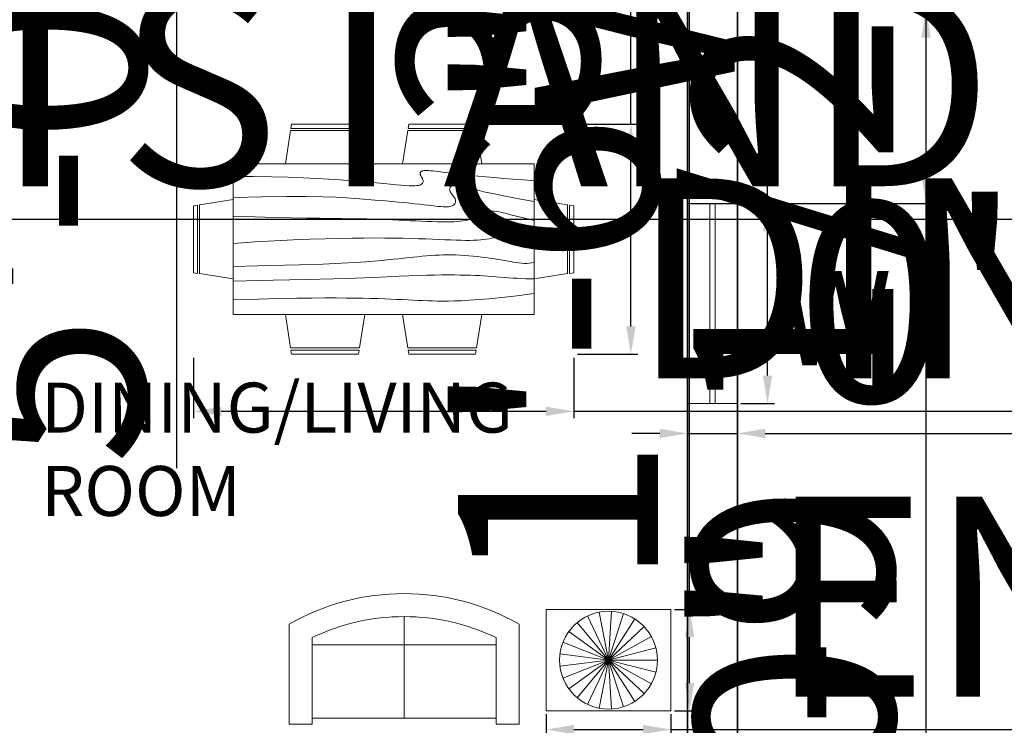
# Model space of a CAD drawing. Units: inches. Extents: x 2901 to 21549, y 2042 to 3828.
# Tile 5 of 10: x 3505 to 3682, y 3099 to 3226. Entities that reach past the tile are written whole.
import ezdxf

# ---------------------------------------------------------------- set-up
doc = ezdxf.new("R2010")
doc.units = ezdxf.units.IN
doc.layers.get('Defpoints').update_dxf_attribs({"color": 1})
for name, color, linetype, lineweight in [('A-ANNO-DIMS', 2, 'Continuous', 18), ('A-ANNO-TEXT', 7, 'Continuous', 18), ('A-AREA-IDEN', 7, 'Continuous', 18), ('A-FURN', 8, 'Continuous', 18), ('A-GLAZ', 4, 'Continuous', 18), ('A-WALL', 7, 'Continuous', 35)]:
    doc.layers.add(name, color=color, linetype=linetype, lineweight=lineweight)
doc.styles.get("Standard").update_dxf_attribs({"font": 'arial.ttf'})
doc.dimstyles.new('ISO-25', dxfattribs={"dimtxt": 36, "dimasz": 5, "dimexe": 1.25, "dimexo": 0.625, "dimtad": 1, "dimdec": 0, "dimlunit": 3, "dimtxsty": 'Standard', "dimcen": 2.5, "dimadec": 0, "dimazin": 0, "dimtfac": 1, "dimtdec": 0, "dimtmove": 0, "dimatfit": 3, "dimfxl": 1, "dimarcsym": 0})

# ---------------------------------------------------------------- blocks, each defined once
blk = doc.blocks.new('Dining Set - 36 x 72 in.')
for p, q in [((-22.2343, 26.00059), (-23.4847, 17.99762)), ((-22.2304, 26), (-5.7608, 26)), ((-22, 27.5), (-22.1562, 26.50042)), ((-5.8416, 26.5), (-22.1534, 26.5)), ((-22, 27.5), (-6, 27.5)), ((-5.8437, 26.49966), (-6, 27.5)), ((-4.5152, 17.99762), (-5.7655, 25.99926)), ((5.7657, 26.00059), (4.5153, 17.99762)), ((5.7696, 26), (22.2392, 26)), ((6, 27.5), (5.8438, 26.50042)), ((22.1584, 26.5), (5.8466, 26.5)), ((6, 27.5), (22, 27.5)), ((22.1563, 26.49966), (22, 27.5)), ((23.4848, 17.99762), (22.2345, 25.99926)), ((36, 18), (-36, 18)), ((-36, 18), (-36, -18)), ((36, -18), (36, 18)), ((-44.0006, 8.23428), (-35.9976, 9.48474)), ((44.0006, 8.23428), (35.9976, 9.48474)), ((-45.5, 8), (-44.5004, 8.15617)), ((-45.5, 8), (-45.5, -8)), ((-44.5, -8.15843), (-44.5, 8.15338)), ((-44, 8.23041), (-44, -8.23915)), ((44, 8.23041), (44, -8.23915)), ((44.5, -8.15843), (44.5, 8.15338)), ((45.5, 8), (44.5005, 8.15617)), ((45.5, 8), (45.5, -8)), ((-44.4997, -8.15631), (-45.5, -8)), ((-35.9976, -9.48476), (-43.9993, -8.2345)), ((35.9976, -9.48476), (43.9993, -8.2345)), ((44.4997, -8.15631), (45.5, -8)), ((-36, -18), (36, -18)), ((-22.2343, -26.0006), (-23.4847, -17.99762)), ((-4.5152, -17.99762), (-5.7655, -25.99928)), ((5.7657, -26.0006), (4.5153, -17.99762)), ((23.4848, -17.99762), (22.2345, -25.99928)), ((-22.2304, -26), (-5.7608, -26)), ((-22, -27.5), (-22.1562, -26.50044)), ((-5.8416, -26.5), (-22.1534, -26.5)), ((-22, -27.5), (-6, -27.5)), ((-5.8437, -26.49967), (-6, -27.5)), ((5.7696, -26), (22.2392, -26)), ((6, -27.5), (5.8438, -26.50044)), ((22.1584, -26.5), (5.8466, -26.5)), ((6, -27.5), (22, -27.5)), ((22.1563, -26.49967), (22, -27.5))]:
    blk.add_line(p, q)
for points in [[(-36, 15), (-31.1772, 14.97754), (-26.8079, 14.91406), (-22.8538, 14.81543), (-19.276, 14.6875), (-16.0362, 14.53613), (-13.0957, 14.36718), (-10.4159, 14.18652), (-7.9583, 14), (-5.6904, 13.81315), (-3.6035, 13.63021), (-1.6954, 13.45508), (0.0365, 13.29166), (1.5945, 13.14388), (2.9811, 13.01562), (4.1988, 12.9108), (5.25, 12.83333), (6.1393, 12.78613), (6.8802, 12.76823), (7.4883, 12.77767), (7.9792, 12.8125), (8.3685, 12.87077), (8.6719, 12.95052), (8.9049, 13.0498), (9.0833, 13.16666), (9.2205, 13.29899), (9.3216, 13.44401), (9.3895, 13.59879), (9.4271, 13.76041), (9.4373, 13.92594), (9.4232, 14.09245), (9.3875, 14.257), (9.3333, 14.41666), (9.2638, 14.56917), (9.1836, 14.71484), (9.0975, 14.85465), (9.0104, 14.98958), (8.9272, 15.1206), (8.8529, 15.2487), (8.7922, 15.37483), (8.75, 15.5), (8.7305, 15.62467), (8.7344, 15.74739), (8.7617, 15.86621), (8.8125, 15.97916), (8.8867, 16.08431), (8.9844, 16.17968), (9.1055, 16.26334), (9.25, 16.33333), (9.4189, 16.38802), (9.6172, 16.42708), (9.8506, 16.45052), (10.125, 16.45833), (10.4463, 16.45052), (10.8203, 16.42708), (11.2529, 16.38802), (11.75, 16.33333), (12.3184, 16.26318), (12.9694, 16.17838), (13.7151, 16.07991), (14.5677, 15.96875), (15.5395, 15.84586), (16.6426, 15.71224), (17.8893, 15.56884), (19.2917, 15.41666), (20.859, 15.25667), (22.5879, 15.08984), (24.4721, 14.91715), (26.5052, 14.73958), (28.6809, 14.5581), (30.9929, 14.3737), (33.4347, 14.18733), (36, 14)], [(-36, 10), (-28.9766, 10.14274), (-23.1725, 10.20442), (-18.4241, 10.19775), (-14.5677, 10.13541), (-11.4399, 10.03011), (-8.877, 9.89453), (-6.7154, 9.74137), (-4.7917, 9.58333), (-2.9698, 9.43082), (-1.2246, 9.28515), (0.4415, 9.14534), (2.026, 9.01041), (3.5266, 8.87939), (4.9408, 8.7513), (6.266, 8.62516), (7.5, 8.5), (8.6411, 8.37549), (9.6914, 8.2539), (10.6538, 8.13818), (11.5312, 8.03125), (12.3267, 7.93603), (13.043, 7.85547), (13.6831, 7.79248), (14.25, 7.75), (14.7471, 7.7303), (15.1797, 7.73307), (15.5537, 7.75732), (15.875, 7.80208), (16.1494, 7.86637), (16.3828, 7.94922), (16.5811, 8.04964), (16.75, 8.16666), (16.8944, 8.29915), (17.0143, 8.44531), (17.1089, 8.60319), (17.1771, 8.77083), (17.218, 8.94629), (17.2305, 9.1276), (17.2137, 9.31282), (17.1667, 9.5), (17.0895, 9.6875), (16.987, 9.875), (16.8649, 10.0625), (16.7292, 10.25), (16.5856, 10.4375), (16.4401, 10.625), (16.2985, 10.8125), (16.1667, 11), (16.05, 11.18733), (15.9518, 11.3737), (15.8752, 11.5581), (15.8229, 11.73958), (15.798, 11.91715), (15.8034, 12.08984), (15.842, 12.25667), (15.9167, 12.41666), (16.0295, 12.56836), (16.1784, 12.70833), (16.3605, 12.83268), (16.5729, 12.9375), (16.8127, 13.01888), (17.0768, 13.07291), (17.3625, 13.0957), (17.6667, 13.08333), (17.9894, 13.03312), (18.3418, 12.94726), (18.7382, 12.82918), (19.1927, 12.68229), (19.7195, 12.51001), (20.3327, 12.31575), (21.0465, 12.10294), (21.875, 11.875), (22.8357, 11.63354), (23.959, 11.37304), (25.2786, 11.08618), (26.8282, 10.76562), (28.6414, 10.40405), (30.752, 9.99414), (33.1936, 9.52856), (36, 9)], [(-36, 5.5), (-30.7157, 5.3348), (-26.069, 5.20963), (-21.9946, 5.11767), (-18.4271, 5.05208), (-15.3009, 5.00602), (-12.5508, 4.97265), (-10.1112, 4.94515), (-7.9167, 4.91666), (-5.909, 4.88167), (-4.0586, 4.83984), (-2.3429, 4.79215), (-0.7396, 4.73958), (0.7739, 4.6831), (2.22, 4.6237), (3.6213, 4.56233), (5, 4.5), (6.373, 4.43782), (7.7344, 4.3776), (9.0723, 4.32129), (10.375, 4.27083), (11.6309, 4.22819), (12.8281, 4.19531), (13.9551, 4.17415), (15, 4.16666), (15.954, 4.17448), (16.819, 4.19791), (17.6001, 4.23698), (18.3021, 4.29166), (18.9299, 4.36198), (19.4883, 4.44791), (19.9823, 4.54948), (20.4167, 4.66666), (20.7969, 4.79899), (21.1302, 4.94401), (21.4245, 5.09879), (21.6875, 5.26041), (21.9271, 5.42594), (22.1511, 5.59245), (22.3672, 5.757), (22.5834, 5.91666), (22.8065, 6.06868), (23.0404, 6.21093), (23.2879, 6.34147), (23.5521, 6.45833), (23.8358, 6.55957), (24.142, 6.64323), (24.4735, 6.70735), (24.8334, 6.75), (25.2235, 6.76969), (25.642, 6.76692), (26.0858, 6.74267), (26.5521, 6.69791), (27.0379, 6.63362), (27.5404, 6.55078), (28.0565, 6.45036), (28.5834, 6.33333), (29.1242, 6.19987), (29.7071, 6.04687), (30.3661, 5.87044), (31.1354, 5.66666), (32.0493, 5.43164), (33.142, 5.16146), (34.4475, 4.85221), (36, 4.5)], [(-36, -1), (-30.7915, -0.6591), (-26.0195, -0.38216), (-21.6519, -0.16284), (-17.6563, 0.00521), (-14.0005, 0.12833), (-10.6523, 0.21289), (-7.5796, 0.26522), (-4.75, 0.29166), (-2.134, 0.29793), (0.2878, 0.28711), (2.5317, 0.26163), (4.6146, 0.22396), (6.5529, 0.17651), (8.3633, 0.12174), (10.0623, 0.06209), (11.6667, 0), (13.1899, -0.06201), (14.6341, -0.1211), (15.9982, -0.17432), (17.2813, -0.21875), (18.4823, -0.25147), (19.6003, -0.26953), (20.6343, -0.27002), (21.5834, -0.25), (22.4481, -0.20768), (23.2357, -0.14584), (23.9549, -0.06836), (24.6146, 0.02083), (25.2235, 0.11784), (25.7904, 0.21875), (26.3241, 0.31966), (26.8334, 0.41666), (27.3265, 0.50618), (27.8099, 0.58593), (28.2894, 0.65397), (28.7709, 0.70833), (29.2601, 0.74707), (29.763, 0.76823), (30.2855, 0.76985), (30.8334, 0.75), (31.4088, 0.70784), (31.9994, 0.64713), (32.589, 0.57275), (33.1615, 0.48958), (33.7008, 0.4025), (34.1908, 0.3164), (34.6153, 0.23616), (34.9584, 0.16666), (35.2099, 0.11165), (35.3848, 0.07031), (35.504, 0.04069), (35.5886, 0.02083), (35.6594, 0.00879), (35.7377, 0.0026), (35.8442, 0.00032), (36, 0)], [(-36, -6.5), (-27.1843, -6.31267), (-20.084, -6.1263), (-14.469, -5.9419), (-10.1094, -5.76042), (-6.7752, -5.58285), (-4.2363, -5.41016), (-2.2629, -5.24333), (-0.625, -5.08334), (0.8708, -4.93099), (2.2715, -4.78646), (3.5872, -4.64974), (4.8281, -4.52084), (6.0046, -4.39974), (7.127, -4.28646), (8.2053, -4.18099), (9.25, -4.08334), (10.2705, -3.99382), (11.2734, -3.91407), (12.2647, -3.84603), (13.25, -3.79167), (14.2354, -3.75293), (15.2266, -3.73177), (16.2295, -3.73015), (17.25, -3.75), (18.2912, -3.79248), (19.3451, -3.85547), (20.4009, -3.93604), (21.4479, -4.03125), (22.4754, -4.13819), (23.4727, -4.25391), (24.4289, -4.37549), (25.3334, -4.5), (26.1785, -4.62492), (26.9694, -4.74935), (27.7145, -4.87281), (28.4219, -4.99479), (29.1, -5.11483), (29.7572, -5.23242), (30.4016, -5.34709), (31.0417, -5.45834), (31.6837, -5.56437), (32.3262, -5.65821), (32.9658, -5.73153), (33.599, -5.77604), (34.2224, -5.78345), (34.8327, -5.74545), (35.4264, -5.65373), (36, -5.5)], [(-36, -10), (-26.4022, -9.81299), (-18.4675, -9.62891), (-11.9839, -9.45069), (-6.7396, -9.28125), (-2.5226, -9.12354), (0.8789, -8.98047), (3.6769, -8.85498), (6.0833, -8.75), (8.2767, -8.66765), (10.3021, -8.60677), (12.1712, -8.56543), (13.8958, -8.54167), (15.4876, -8.53353), (16.9583, -8.53907), (18.3197, -8.55632), (19.5834, -8.58334), (20.7616, -8.61841), (21.8685, -8.66081), (22.9188, -8.71004), (23.9271, -8.76563), (24.9081, -8.82707), (25.8763, -8.89388), (26.8465, -8.96558), (27.8334, -9.04167), (28.8474, -9.12118), (29.8828, -9.20117), (30.93, -9.27824), (31.9792, -9.34896), (33.0205, -9.40991), (34.0443, -9.45768), (35.0407, -9.48885), (36, -9.5)], [(-36, -14.5), (-30.0881, -14.33513), (-25.0332, -14.21224), (-20.7312, -14.12647), (-17.0781, -14.07292), (-13.97, -14.04671), (-11.3027, -14.04297), (-8.9724, -14.05681), (-6.875, -14.08334), (-4.9224, -14.11833), (-3.0905, -14.16016), (-1.3709, -14.20785), (0.2448, -14.26042), (1.7647, -14.3169), (3.1973, -14.3763), (4.5507, -14.43767), (5.8333, -14.5), (7.0554, -14.5621), (8.235, -14.62175), (9.3922, -14.67652), (10.5469, -14.72396), (11.7192, -14.76164), (12.929, -14.78711), (14.1965, -14.79794), (15.5417, -14.79167), (16.9933, -14.76424), (18.6152, -14.70508), (20.4804, -14.60197), (22.6615, -14.44271), (25.2312, -14.21509), (28.2624, -13.9069), (31.8277, -13.50594), (36, -13)]]:
    blk.add_lwpolyline(points)
blk = doc.blocks.new('Sofa - Roundback Loveseat 5 ft.')
for p, q in [((0, -32.44198), (0, -5.99998)), ((-24, -33.99998), (-24, -11.46958)), ((24.00004, -33.99998), (24.00004, -11.46958)), ((-23.9998, -13.38178), (23.99986, -13.38178)), ((-24, -32.44198), (24.00004, -32.44198))]:
    blk.add_line(p, q)
for points in [[(-24, -33.99998), (-30, -33.99998), (-30, -7.99998)], [(30.00004, -7.99998), (30.00004, -33.99998), (24.00004, -33.99998)]]:
    blk.add_lwpolyline(points)
for centre, radius, start, end in [((0, -60.24998), 60.24998, 60.13715, 119.8628), ((0, -61.38438), 55.38444, 64.32083, 115.6792)]:
    blk.add_arc(centre, radius, start, end)
blk = doc.blocks.new('WIN-36IN-9IN-WALL')
for p, q in [((0, 36), (9, 36)), ((0, 0), (0, 36)), ((4, 0), (4, 36)), ((5, 36), (5, 0)), ((9, 36), (9, 0)), ((9, 0), (0, 0))]:
    blk.add_line(p, q)
blk = doc.blocks.new('*U24')
blk.add_line((-4.41, 0), (4.41, 0))
blk = doc.blocks.new('*U25')
at = {"color": 0, "linetype": 'ByBlock', "lineweight": -2, "transparency": 16777216}
for p, rotation in [((3610.1, 3028.89), 100.7999999999996), ((3611.21, 3028.96), 86.39999999999972), ((3612.29, 3028.76), 71.99999999999977), ((3608.12, 3027.96), 129.5999999999996), ((3609.05, 3028.55), 115.1999999999997), ((3613.29, 3028.29), 57.59999999999982), ((3607.36, 3027.15), 143.9999999999996), ((3614.14, 3027.58), 43.19999999999986), ((3606.83, 3026.19), 158.3999999999996), ((3614.79, 3026.69), 28.7999999999999), ((3615.2, 3025.66), 14.39999999999998), ((3606.56, 3025.12), 172.7999999999996), ((3606.56, 3024.01), 187.1999999999994), ((3606.83, 3022.94), 201.5999999999995), ((3607.36, 3021.97), 215.9999999999995), ((3608.12, 3021.17), 230.3999999999995), ((3609.05, 3020.58), 244.7999999999995), ((3610.1, 3020.23), 259.1999999999994), ((3611.21, 3020.17), 273.5999999999994), ((3612.29, 3020.37), 287.9999999999993), ((3613.29, 3020.84), 302.3999999999992), ((3614.14, 3021.55), 316.7999999999993), ((3614.79, 3022.44), 331.1999999999992), ((3615.2, 3023.47), 345.5999999999992)]:
    blk.add_blockref('*U24', p, dxfattribs=dict(at, rotation=rotation))
blk.add_blockref('*U24', (3615.34, 3024.56), dxfattribs=at)
blk = doc.blocks.new('TABLE-END-DECOR')
blk.add_lwpolyline([(0, 18.24), (22.47, 18.24), (22.47, 0), (0, 0)], close=True)
blk.add_circle((11.23, 9.12), 8.81)
blk.add_blockref('*U25', (-3599.7, -3015.44))
blk = doc.blocks.new('*D36')
at = {"layer": 'A-ANNO-DIMS', "color": 0, "lineweight": -2, "transparency": 16777216}
for p, q in [((3639.47, 3192.64), (3639.47, 3654.44)), ((3634.69, 3192.64), (3640.72, 3192.64)), ((3639.47, 3161.64), (3639.47, 3187.64)), ((3634.69, 3156.64), (3640.72, 3156.64))]:
    blk.add_line(p, q, dxfattribs=at)
at = {"layer": 'A-ANNO-DIMS', "color": 0, "transparency": 16777216}
for points in [[(3638.64, 3187.64), (3640.3, 3187.64), (3639.47, 3192.64)], [(3638.64, 3161.64), (3640.3, 3161.64), (3639.47, 3156.64)]]:
    blk.add_solid(points, dxfattribs=at)
at = {"layer": 'Defpoints', "color": 0, "transparency": 16777216}
for p in [(3634.07, 3192.64), (3639.47, 3192.64), (3634.07, 3156.64)]:
    blk.add_point(p, dxfattribs=at)
at = {"layer": 'A-ANNO-DIMS', "color": 0, "transparency": 16777216, "insert": (3620.21, 3426.04), "char_height": 36, "attachment_point": 5, "rotation": 90}
blk.add_mtext('WINDOW 3\'-0" TYP.', dxfattribs=at)
blk = doc.blocks.new('*D37')
at = {"layer": 'A-ANNO-DIMS', "color": 0, "lineweight": -2, "transparency": 16777216}
for p, q in [((3625.07, 3156.01), (3625.07, 3149.99)), ((3634.07, 3156.01), (3634.07, 3149.99)), ((3620.07, 3151.24), (3615.07, 3151.24)), ((3625.07, 3151.24), (3634.07, 3151.24)), ((3639.07, 3151.24), (3864.76, 3151.24))]:
    blk.add_line(p, q, dxfattribs=at)
at = {"layer": 'A-ANNO-DIMS', "color": 0, "transparency": 16777216}
for points in [[(3620.07, 3152.07), (3620.07, 3150.41), (3625.07, 3151.24)], [(3639.07, 3152.07), (3639.07, 3150.41), (3634.07, 3151.24)]]:
    blk.add_solid(points, dxfattribs=at)
at = {"layer": 'Defpoints', "color": 0, "transparency": 16777216}
for p in [(3625.07, 3156.64), (3634.07, 3156.64), (3634.07, 3151.24)]:
    blk.add_point(p, dxfattribs=at)
at = {"layer": 'A-ANNO-DIMS', "color": 0, "transparency": 16777216, "insert": (3754.41, 3170.24), "char_height": 36, "attachment_point": 5}
blk.add_mtext('0\'-9" TYP.', dxfattribs=at)
blk = doc.blocks.new('*D38')
at = {"layer": 'A-ANNO-DIMS', "color": 0, "lineweight": -2, "transparency": 16777216}
for p, q in [((3343.07, 3191.34), (3343.07, 3188.58)), ((3357.29, 3191.34), (3357.29, 3188.58)), ((3348.07, 3189.83), (3352.29, 3189.83)), ((3357.29, 3189.83), (3922.11, 3189.83))]:
    blk.add_line(p, q, dxfattribs=at)
at = {"layer": 'A-ANNO-DIMS', "color": 0, "transparency": 16777216}
for points in [[(3348.07, 3190.67), (3348.07, 3189), (3343.07, 3189.83)], [(3352.29, 3190.67), (3352.29, 3189), (3357.29, 3189.83)]]:
    blk.add_solid(points, dxfattribs=at)
at = {"layer": 'Defpoints', "color": 0, "transparency": 16777216}
for p in [(3343.07, 3191.97), (3357.29, 3191.97), (3357.29, 3189.83)]:
    blk.add_point(p, dxfattribs=at)
at = {"layer": 'A-ANNO-DIMS', "color": 0, "transparency": 16777216, "insert": (3642.2, 3209.07), "char_height": 36, "attachment_point": 5}
blk.add_mtext('NIGHTSTAND 1\'-2" TYP.', dxfattribs=at)
blk = doc.blocks.new('*D43')
at = {"layer": 'A-ANNO-DIMS', "color": 0, "lineweight": -2, "transparency": 16777216}
for p, q in [((3550.8, 3269.4), (3856.95, 3274.04)), ((3536.1, 3267.11), (3536.05, 3270.42)), ((3550.83, 3267.33), (3550.78, 3270.65)), ((3541.07, 3269.25), (3545.8, 3269.32))]:
    blk.add_line(p, q, dxfattribs=at)
at = {"layer": 'A-ANNO-DIMS', "color": 0, "transparency": 16777216}
for points in [[(3541.06, 3270.08), (3541.09, 3268.42), (3536.07, 3269.17)], [(3545.78, 3270.16), (3545.81, 3268.49), (3550.8, 3269.4)]]:
    blk.add_solid(points, dxfattribs=at)
at = {"layer": 'Defpoints', "color": 0, "transparency": 16777216}
for p in [(3550.8, 3269.4), (3536.11, 3266.48), (3550.84, 3266.71)]:
    blk.add_point(p, dxfattribs=at)
at = {"layer": 'A-ANNO-DIMS', "color": 0, "transparency": 16777216, "insert": (3706.08, 3290.99), "char_height": 36, "attachment_point": 5, "rotation": 0.8679}
blk.add_mtext('1\'-2 1/2" TYP.', dxfattribs=at)
blk = doc.blocks.new('*D47')
at = {"layer": 'A-ANNO-DIMS', "color": 0, "lineweight": -2, "transparency": 16777216}
for p, q in [((3544.44, 3430.67), (3531.82, 3430.67)), ((3533.07, 3425.67), (3533.07, 3375.67)), ((3544.44, 3370.67), (3531.82, 3370.67)), ((3533.07, 3370.67), (3533.07, 3144.99))]:
    blk.add_line(p, q, dxfattribs=at)
at = {"layer": 'A-ANNO-DIMS', "color": 0, "transparency": 16777216}
for points in [[(3532.24, 3425.67), (3533.9, 3425.67), (3533.07, 3430.67)], [(3532.24, 3375.67), (3533.9, 3375.67), (3533.07, 3370.67)]]:
    blk.add_solid(points, dxfattribs=at)
at = {"layer": 'Defpoints', "color": 0, "transparency": 16777216}
for p in [(3545.07, 3430.67), (3533.07, 3370.67), (3545.07, 3370.67)]:
    blk.add_point(p, dxfattribs=at)
at = {"layer": 'A-ANNO-DIMS', "color": 0, "transparency": 16777216, "insert": (3514.06, 3255.33), "char_height": 36, "attachment_point": 5, "rotation": 90}
blk.add_mtext('5\'-0" TYP.', dxfattribs=at)
blk = doc.blocks.new('*D48')
at = {"layer": 'A-ANNO-DIMS', "color": 0, "lineweight": -2, "transparency": 16777216}
for p, q in [((3552.33, 3036.58), (3552.33, 3043.43)), ((3557.33, 3042.18), (3588.77, 3042.18)), ((3593.77, 3036.58), (3593.77, 3043.43)), ((3593.77, 3042.18), (4181.25, 3042.18))]:
    blk.add_line(p, q, dxfattribs=at)
at = {"layer": 'A-ANNO-DIMS', "color": 0, "transparency": 16777216}
for points in [[(3557.33, 3043.01), (3557.33, 3041.34), (3552.33, 3042.18)], [(3588.77, 3043.01), (3588.77, 3041.34), (3593.77, 3042.18)]]:
    blk.add_solid(points, dxfattribs=at)
at = {"layer": 'Defpoints', "color": 0, "transparency": 16777216}
for p in [(3593.77, 3042.18), (3552.33, 3035.96), (3593.77, 3035.96)]:
    blk.add_point(p, dxfattribs=at)
at = {"layer": 'A-ANNO-DIMS', "color": 0, "transparency": 16777216, "insert": (3890.01, 3061.44), "char_height": 36, "attachment_point": 5}
blk.add_mtext('LOVESEAT 3\'-5 1/2" TYP.', dxfattribs=at)
blk = doc.blocks.new('*D50')
at = {"layer": 'A-ANNO-DIMS', "color": 0, "lineweight": -2, "transparency": 16777216}
for p, q in [((3599.61, 3100.68), (3599.61, 3096.69)), ((3622.08, 3100.68), (3622.08, 3096.69)), ((3604.61, 3097.94), (3617.08, 3097.94)), ((3622.08, 3097.94), (4251.18, 3097.94))]:
    blk.add_line(p, q, dxfattribs=at)
at = {"layer": 'A-ANNO-DIMS', "color": 0, "transparency": 16777216}
for points in [[(3604.61, 3098.77), (3604.61, 3097.1), (3599.61, 3097.94)], [(3617.08, 3098.77), (3617.08, 3097.1), (3622.08, 3097.94)]]:
    blk.add_solid(points, dxfattribs=at)
at = {"layer": 'Defpoints', "color": 0, "transparency": 16777216}
for p in [(3599.61, 3101.31), (3622.08, 3101.31), (3622.08, 3097.94)]:
    blk.add_point(p, dxfattribs=at)
at = {"layer": 'A-ANNO-DIMS', "color": 0, "transparency": 16777216, "insert": (3939.13, 3117.18), "char_height": 36, "attachment_point": 5}
blk.add_mtext('END TABLE 1\'-10 1/2" TYP.', dxfattribs=at)
blk = doc.blocks.new('*D51')
at = {"layer": 'A-ANNO-DIMS', "color": 0, "lineweight": -2, "transparency": 16777216}
for p, q in [((3625.45, 3119.55), (3625.45, 3341.85)), ((3622.7, 3119.55), (3626.7, 3119.55)), ((3625.45, 3106.31), (3625.45, 3114.55)), ((3622.7, 3101.31), (3626.7, 3101.31))]:
    blk.add_line(p, q, dxfattribs=at)
at = {"layer": 'A-ANNO-DIMS', "color": 0, "transparency": 16777216}
for points in [[(3624.61, 3114.55), (3626.28, 3114.55), (3625.45, 3119.55)], [(3624.61, 3106.31), (3626.28, 3106.31), (3625.45, 3101.31)]]:
    blk.add_solid(points, dxfattribs=at)
at = {"layer": 'Defpoints', "color": 0, "transparency": 16777216}
for p in [(3622.08, 3119.55), (3625.45, 3119.55), (3622.08, 3101.31)]:
    blk.add_point(p, dxfattribs=at)
at = {"layer": 'A-ANNO-DIMS', "color": 0, "transparency": 16777216, "insert": (3606.44, 3233.2), "char_height": 36, "attachment_point": 5, "rotation": 90}
blk.add_mtext('1\'-6" TYP.', dxfattribs=at)
blk = doc.blocks.new('*D52')
at = {"layer": 'A-ANNO-DIMS', "color": 0, "lineweight": -2, "transparency": 16777216}
for p, q in [((3469.26, 3197.35), (3456.81, 3197.35)), ((3458.06, 3192.35), (3458.06, 3123.52)), ((3469.26, 3118.52), (3456.81, 3118.52)), ((3458.06, 3118.52), (3458.06, 2589.92))]:
    blk.add_line(p, q, dxfattribs=at)
at = {"layer": 'A-ANNO-DIMS', "color": 0, "transparency": 16777216}
for points in [[(3457.23, 3192.35), (3458.9, 3192.35), (3458.06, 3197.35)], [(3457.23, 3123.52), (3458.9, 3123.52), (3458.06, 3118.52)]]:
    blk.add_solid(points, dxfattribs=at)
at = {"layer": 'Defpoints', "color": 0, "transparency": 16777216}
for p in [(3469.89, 3197.35), (3458.06, 3118.52), (3469.89, 3118.52)]:
    blk.add_point(p, dxfattribs=at)
at = {"layer": 'A-ANNO-DIMS', "color": 0, "transparency": 16777216, "insert": (3439.06, 2851.72), "char_height": 36, "attachment_point": 5, "rotation": 90}
blk.add_mtext('MEDIA UNIT 6\'-7" TYP.', dxfattribs=at)
blk = doc.blocks.new('*D54')
at = {"layer": 'A-ANNO-DIMS', "color": 0, "lineweight": -2, "transparency": 16777216}
for p, q in [((3536.12, 3164.87), (3536.12, 3153.97)), ((3604.61, 3164.87), (3604.61, 3153.97)), ((3541.12, 3155.22), (3599.61, 3155.22)), ((3604.61, 3155.22), (4090.43, 3155.22))]:
    blk.add_line(p, q, dxfattribs=at)
at = {"layer": 'A-ANNO-DIMS', "color": 0, "transparency": 16777216}
for points in [[(3541.12, 3156.05), (3541.12, 3154.38), (3536.12, 3155.22)], [(3599.61, 3156.05), (3599.61, 3154.38), (3604.61, 3155.22)]]:
    blk.add_solid(points, dxfattribs=at)
at = {"layer": 'Defpoints', "color": 0, "transparency": 16777216}
for p in [(3536.12, 3165.49), (3604.61, 3165.49), (3604.61, 3155.22)]:
    blk.add_point(p, dxfattribs=at)
at = {"layer": 'A-ANNO-DIMS', "color": 0, "transparency": 16777216, "insert": (3850.02, 3174.46), "char_height": 36, "attachment_point": 5}
blk.add_mtext('DINING SET 5\'-8 1/2"', dxfattribs=at)
blk = doc.blocks.new('*D55')
at = {"layer": 'A-ANNO-DIMS', "color": 0, "lineweight": -2, "transparency": 16777216}
for p, q in [((3614.88, 3206.89), (3614.88, 3392.69)), ((3605.24, 3206.89), (3616.13, 3206.89)), ((3614.88, 3170.49), (3614.88, 3201.89)), ((3605.24, 3165.49), (3616.13, 3165.49))]:
    blk.add_line(p, q, dxfattribs=at)
at = {"layer": 'A-ANNO-DIMS', "color": 0, "transparency": 16777216}
for points in [[(3614.05, 3201.89), (3615.72, 3201.89), (3614.88, 3206.89)], [(3614.05, 3170.49), (3615.72, 3170.49), (3614.88, 3165.49)]]:
    blk.add_solid(points, dxfattribs=at)
at = {"layer": 'Defpoints', "color": 0, "transparency": 16777216}
for p in [(3604.61, 3206.89), (3614.88, 3206.89), (3604.61, 3165.49)]:
    blk.add_point(p, dxfattribs=at)
at = {"layer": 'A-ANNO-DIMS', "color": 0, "transparency": 16777216, "insert": (3595.63, 3302.29), "char_height": 36, "attachment_point": 5, "rotation": 90}
blk.add_mtext('3\'-5 1/2"', dxfattribs=at)
blk = doc.blocks.new('*D57')
at = {"layer": 'A-ANNO-DIMS', "color": 0, "lineweight": -2, "transparency": 16777216}
for p, q in [((3601.59, 3038.97), (3601.59, 3029.64)), ((3626.91, 3038.97), (3626.91, 3029.64)), ((3606.59, 3030.89), (3621.91, 3030.89)), ((3626.91, 3030.89), (3813.36, 3030.89))]:
    blk.add_line(p, q, dxfattribs=at)
at = {"layer": 'A-ANNO-DIMS', "color": 0, "transparency": 16777216}
for points in [[(3606.59, 3031.73), (3606.59, 3030.06), (3601.59, 3030.89)], [(3621.91, 3031.73), (3621.91, 3030.06), (3626.91, 3030.89)]]:
    blk.add_solid(points, dxfattribs=at)
at = {"layer": 'Defpoints', "color": 0, "transparency": 16777216}
for p in [(3601.59, 3039.6), (3626.91, 3039.6), (3626.91, 3030.89)]:
    blk.add_point(p, dxfattribs=at)
at = {"layer": 'A-ANNO-DIMS', "color": 0, "transparency": 16777216, "insert": (3722.63, 3050.13), "char_height": 36, "attachment_point": 5}
blk.add_mtext('2\'-1 1/2"', dxfattribs=at)
blk = doc.blocks.new('*D65')
at = {"layer": 'A-ANNO-DIMS', "color": 0, "lineweight": -2, "transparency": 16777216}
for p, q in [((3668.02, 3003.48), (3668.02, 3130.01)), ((3625.69, 3003.48), (3669.27, 3003.48)), ((3668.02, 2888.48), (3668.02, 2998.48)), ((3625.69, 2883.48), (3669.27, 2883.48))]:
    blk.add_line(p, q, dxfattribs=at)
at = {"layer": 'A-ANNO-DIMS', "color": 0, "transparency": 16777216}
for points in [[(3667.19, 2998.48), (3668.85, 2998.48), (3668.02, 3003.48)], [(3667.19, 2888.48), (3668.85, 2888.48), (3668.02, 2883.48)]]:
    blk.add_solid(points, dxfattribs=at)
at = {"layer": 'Defpoints', "color": 0, "transparency": 16777216}
for p in [(3625.07, 3003.48), (3668.02, 3003.48), (3625.07, 2883.48)]:
    blk.add_point(p, dxfattribs=at)
at = {"layer": 'A-ANNO-DIMS', "color": 0, "transparency": 16777216, "insert": (3649.01, 3069.24), "char_height": 36, "attachment_point": 5, "rotation": 90}
blk.add_mtext('10\'-0"', dxfattribs=at)
blk = doc.blocks.new('*D67')
at = {"layer": 'A-ANNO-DIMS', "color": 0, "lineweight": -2, "transparency": 16777216}
for p, q in [((3484.07, 3013.1), (3484.07, 3509.68)), ((3489.07, 3508.43), (3620.07, 3508.43)), ((3625.07, 3228.1), (3625.07, 3509.68))]:
    blk.add_line(p, q, dxfattribs=at)
at = {"layer": 'A-ANNO-DIMS', "color": 0, "transparency": 16777216}
for points in [[(3489.07, 3509.26), (3489.07, 3507.59), (3484.07, 3508.43)], [(3620.07, 3509.26), (3620.07, 3507.59), (3625.07, 3508.43)]]:
    blk.add_solid(points, dxfattribs=at)
at = {"layer": 'Defpoints', "color": 0, "transparency": 16777216}
for p in [(3625.07, 3508.43), (3625.07, 3227.48), (3484.07, 3012.48)]:
    blk.add_point(p, dxfattribs=at)
at = {"layer": 'A-ANNO-DIMS', "color": 0, "transparency": 16777216, "insert": (3554.57, 3527.43), "char_height": 36, "attachment_point": 5}
blk.add_mtext('11\'-9"', dxfattribs=at)
blk = doc.blocks.new('*D68')
at = {"layer": 'A-ANNO-DIMS', "color": 0, "lineweight": -2, "transparency": 16777216}
for p, q in [((3531.44, 3227.48), (3298.87, 3227.48)), ((3300.12, 3017.48), (3300.12, 3222.48)), ((3483.44, 3012.48), (3298.87, 3012.48))]:
    blk.add_line(p, q, dxfattribs=at)
at = {"layer": 'A-ANNO-DIMS', "color": 0, "transparency": 16777216}
for points in [[(3299.29, 3222.48), (3300.95, 3222.48), (3300.12, 3227.48)], [(3299.29, 3017.48), (3300.95, 3017.48), (3300.12, 3012.48)]]:
    blk.add_solid(points, dxfattribs=at)
at = {"layer": 'Defpoints', "color": 0, "transparency": 16777216}
for p in [(3300.12, 3227.48), (3532.07, 3227.48), (3484.07, 3012.48)]:
    blk.add_point(p, dxfattribs=at)
at = {"layer": 'A-ANNO-DIMS', "color": 0, "transparency": 16777216, "insert": (3281.42, 3119.98), "char_height": 36, "attachment_point": 5, "rotation": 90}
blk.add_mtext('17\'-11"', dxfattribs=at)
blk = doc.blocks.new('*D73')
at = {"layer": 'A-ANNO-DIMS', "color": 0, "lineweight": -2, "transparency": 16777216}
for p, q in [((3668.02, 3058.19), (3668.02, 3244)), ((3625.69, 3058.19), (3669.27, 3058.19)), ((3668.02, 3017.48), (3668.02, 3053.19)), ((3625.69, 3012.48), (3669.27, 3012.48))]:
    blk.add_line(p, q, dxfattribs=at)
at = {"layer": 'A-ANNO-DIMS', "color": 0, "transparency": 16777216}
for points in [[(3667.19, 3053.19), (3668.85, 3053.19), (3668.02, 3058.19)], [(3667.19, 3017.48), (3668.85, 3017.48), (3668.02, 3012.48)]]:
    blk.add_solid(points, dxfattribs=at)
at = {"layer": 'Defpoints', "color": 0, "transparency": 16777216}
for p in [(3625.07, 3058.19), (3668.02, 3058.19), (3625.07, 3012.48)]:
    blk.add_point(p, dxfattribs=at)
at = {"layer": 'A-ANNO-DIMS', "color": 0, "transparency": 16777216, "insert": (3648.77, 3153.6), "char_height": 36, "attachment_point": 5, "rotation": 90}
blk.add_mtext('3\'-9 1/2"', dxfattribs=at)
blk = doc.blocks.new('*D74')
at = {"layer": 'A-ANNO-DIMS', "color": 0, "lineweight": -2, "transparency": 16777216}
for p, q in [((3668.02, 3227.48), (3668.02, 3358.01)), ((3625.69, 3227.48), (3669.27, 3227.48)), ((3668.02, 3197.64), (3668.02, 3222.48)), ((3625.69, 3192.64), (3669.27, 3192.64))]:
    blk.add_line(p, q, dxfattribs=at)
at = {"layer": 'A-ANNO-DIMS', "color": 0, "transparency": 16777216}
for points in [[(3667.19, 3222.48), (3668.85, 3222.48), (3668.02, 3227.48)], [(3667.19, 3197.64), (3668.85, 3197.64), (3668.02, 3192.64)]]:
    blk.add_solid(points, dxfattribs=at)
at = {"layer": 'Defpoints', "color": 0, "transparency": 16777216}
for p in [(3625.07, 3227.48), (3668.02, 3227.48), (3625.07, 3192.64)]:
    blk.add_point(p, dxfattribs=at)
at = {"layer": 'A-ANNO-DIMS', "color": 0, "transparency": 16777216, "insert": (3649.32, 3295.24), "char_height": 36, "attachment_point": 5, "rotation": 90}
blk.add_mtext('2\'-11"', dxfattribs=at)
blk = doc.blocks.new('*D78')
at = {"layer": 'A-ANNO-DIMS', "color": 0, "lineweight": -2, "transparency": 16777216}
for p, q in [((3343.07, 3230.85), (3343.07, 2839.28)), ((3366.66, 3230.85), (3366.66, 2839.28)), ((3348.07, 2840.53), (3361.66, 2840.53)), ((3366.66, 2840.53), (3577.07, 2840.53))]:
    blk.add_line(p, q, dxfattribs=at)
at = {"layer": 'A-ANNO-DIMS', "color": 0, "transparency": 16777216}
for points in [[(3348.07, 2841.36), (3348.07, 2839.69), (3343.07, 2840.53)], [(3361.66, 2841.36), (3361.66, 2839.69), (3366.66, 2840.53)]]:
    blk.add_solid(points, dxfattribs=at)
at = {"layer": 'Defpoints', "color": 0, "transparency": 16777216}
for p in [(3343.07, 3231.48), (3366.66, 3231.48), (3366.66, 2840.53)]:
    blk.add_point(p, dxfattribs=at)
at = {"layer": 'A-ANNO-DIMS', "color": 0, "transparency": 16777216, "insert": (3474.37, 2859.77), "char_height": 36, "attachment_point": 5}
blk.add_mtext('1\'-11 1/2"', dxfattribs=at)
blk = doc.blocks.new('*D84')
at = {"layer": 'A-ANNO-DIMS', "color": 0, "lineweight": -2, "transparency": 16777216}
for p, q in [((3444.07, 3230.85), (3444.07, 2839.28)), ((3480.07, 3230.85), (3480.07, 2839.28)), ((3449.07, 2840.53), (3475.07, 2840.53)), ((3480.07, 2840.53), (3581.99, 2840.53))]:
    blk.add_line(p, q, dxfattribs=at)
at = {"layer": 'A-ANNO-DIMS', "color": 0, "transparency": 16777216}
for points in [[(3449.07, 2841.36), (3449.07, 2839.69), (3444.07, 2840.53)], [(3475.07, 2841.36), (3475.07, 2839.69), (3480.07, 2840.53)]]:
    blk.add_solid(points, dxfattribs=at)
at = {"layer": 'Defpoints', "color": 0, "transparency": 16777216}
for p in [(3444.07, 3231.48), (3480.07, 3231.48), (3480.07, 2840.53)]:
    blk.add_point(p, dxfattribs=at)
at = {"layer": 'A-ANNO-DIMS', "color": 0, "transparency": 16777216, "insert": (3533.53, 2859.55), "char_height": 36, "attachment_point": 5}
blk.add_mtext('3\'-0"', dxfattribs=at)

msp = doc.modelspace()

# ---------------------------------------------------------------- linework, layer by layer
at = {"layer": 'A-WALL'}
msp.add_line((3625.07, 3465.48), (3625.07, 2883.48), dxfattribs=at)
msp.add_lwpolyline([(3634.07, 3474.48), (3634.07, 2874.48), (3334.07, 2874.48), (3334.07, 3474.48)], close=True, dxfattribs=at)

# ---------------------------------------------------------------- block references
at = {"layer": 'A-FURN'}
for name, p, xscale, yscale, zscale in [('Dining Set - 36 x 72 in.', (3570.36, 3186.19), 0.7526619359100934, 0.7526619359100934, 0.7526619359100934), ('Sofa - Roundback Loveseat 5 ft.', (3574.05, 3122.41), 0.690663340395338, 0.690663340395338, 0.690663340395338)]:
    msp.add_blockref(name, p, dxfattribs=dict(at, xscale=xscale, yscale=yscale, zscale=zscale))
msp.add_blockref('TABLE-END-DECOR', (3599.61, 3101.31), dxfattribs=at)
at = {"layer": 'A-GLAZ'}
msp.add_blockref('WIN-36IN-9IN-WALL', (3625.07, 3156.64), dxfattribs=at)

# ---------------------------------------------------------------- texts
at = {"layer": 'A-ANNO-TEXT', "insert": (3641.55, 3180.47), "char_height": 17, "attachment_point": 1}
msp.add_mtext_dynamic_manual_height_columns('{\\fArial|b1|i0|c0|p34;W}', width=86.7973, gutter_width=12.5, heights=[27.4], dxfattribs=at)
at = {"layer": 'A-AREA-IDEN', "insert": (3508.7, 3160.38), "char_height": 9, "attachment_point": 1}
msp.add_mtext_dynamic_manual_height_columns('{\\fArial|b1|i0|c0|p34;DINING/LIVING ROOM}', width=101.8112, gutter_width=12.5, heights=[34.38], dxfattribs=at)

# ---------------------------------------------------------------- dimensions: what is measured, and where the dimension line sits
at = {"layer": 'A-ANNO-DIMS'}
for base, p1, p2, angle, text, picture, middle in [((3639.47, 3192.64), (3634.07, 3156.64), (3634.07, 3192.64), 90, 'WINDOW <> TYP.', '*D36', (3620.21, 3426.04)), ((3533.07, 3370.67), (3545.07, 3430.67), (3545.07, 3370.67), 270, '<> TYP.', '*D47', (3514.06, 3255.33)), ((3550.8, 3269.4), (3536.11, 3266.48), (3550.84, 3266.71), 0.8679, '<> TYP.', '*D43', (3706.08, 3290.99)), ((3625.45, 3119.55), (3622.08, 3101.31), (3622.08, 3119.55), 90, '<> TYP.', '*D51', (3606.44, 3233.2)), ((3458.06, 3118.52), (3469.89, 3197.35), (3469.89, 3118.52), 270, 'MEDIA UNIT <> TYP.', '*D52', (3439.06, 2851.72))]:
    dim = msp.add_linear_dim(base=base, p1=p1, p2=p2, angle=angle, text=text, dimstyle='ISO-25', override={"dimdec": 1, "dimlfac": 1, "dimrnd": 0, "dimzin": 1, "dimdsep": 46, "dimlunit": 4, "dimfrac": 2}, dxfattribs=at)
    dim.commit()
    dim.dimension.update_dxf_attribs({"geometry": picture, "text_midpoint": middle})
for base, p1, p2, picture, middle in [((3625.07, 3508.43), (3484.07, 3012.48), (3625.07, 3227.48), '*D67', (3554.57, 3527.43)), ((3366.66, 2840.53), (3343.07, 3231.48), (3366.66, 3231.48), '*D78', (3474.37, 2859.77)), ((3480.07, 2840.53), (3444.07, 3231.48), (3480.07, 3231.48), '*D84', (3533.53, 2859.55)), ((3626.91, 3030.89), (3601.59, 3039.6), (3626.91, 3039.6), '*D57', (3722.63, 3050.13))]:
    dim = msp.add_linear_dim(base=base, p1=p1, p2=p2, dimstyle='ISO-25', override={"dimdec": 1, "dimlfac": 1, "dimrnd": 0, "dimzin": 1, "dimdsep": 46, "dimlunit": 4, "dimfrac": 2}, dxfattribs=at)
    dim.commit()
    dim.dimension.update_dxf_attribs({"geometry": picture, "text_midpoint": middle})
for base, p1, p2, picture, middle in [((3614.88, 3206.89), (3604.61, 3165.49), (3604.61, 3206.89), '*D55', (3595.63, 3302.29)), ((3668.02, 3227.48), (3625.07, 3192.64), (3625.07, 3227.48), '*D74', (3649.32, 3295.24)), ((3668.02, 3058.19), (3625.07, 3012.48), (3625.07, 3058.19), '*D73', (3648.77, 3153.6)), ((3300.12, 3227.48), (3484.07, 3012.48), (3532.07, 3227.48), '*D68', (3281.42, 3119.98)), ((3668.02, 3003.48), (3625.07, 2883.48), (3625.07, 3003.48), '*D65', (3649.01, 3069.24))]:
    dim = msp.add_linear_dim(base=base, p1=p1, p2=p2, angle=90, dimstyle='ISO-25', override={"dimdec": 1, "dimlfac": 1, "dimrnd": 0, "dimzin": 1, "dimdsep": 46, "dimlunit": 4, "dimfrac": 2}, dxfattribs=at)
    dim.commit()
    dim.dimension.update_dxf_attribs({"geometry": picture, "text_midpoint": middle})
for base, p1, p2, text, picture, middle in [((3357.29, 3189.83), (3343.07, 3191.97), (3357.29, 3191.97), 'NIGHTSTAND <> TYP.', '*D38', (3642.2, 3209.07)), ((3604.61, 3155.22), (3536.12, 3165.49), (3604.61, 3165.49), 'DINING SET <>', '*D54', (3850.02, 3174.46)), ((3622.08, 3097.94), (3599.61, 3101.31), (3622.08, 3101.31), 'END TABLE <> TYP.', '*D50', (3939.13, 3117.18)), ((3634.07, 3151.24), (3625.07, 3156.64), (3634.07, 3156.64), '<> TYP.', '*D37', (3754.41, 3170.24)), ((3593.77, 3042.18), (3552.33, 3035.96), (3593.77, 3035.96), 'LOVESEAT <> TYP.', '*D48', (3890.01, 3061.44))]:
    dim = msp.add_linear_dim(base=base, p1=p1, p2=p2, text=text, dimstyle='ISO-25', override={"dimdec": 1, "dimlfac": 1, "dimrnd": 0, "dimzin": 1, "dimdsep": 46, "dimlunit": 4, "dimfrac": 2}, dxfattribs=at)
    dim.commit()
    dim.dimension.update_dxf_attribs({"geometry": picture, "text_midpoint": middle})

doc.saveas('drawing.dxf')
